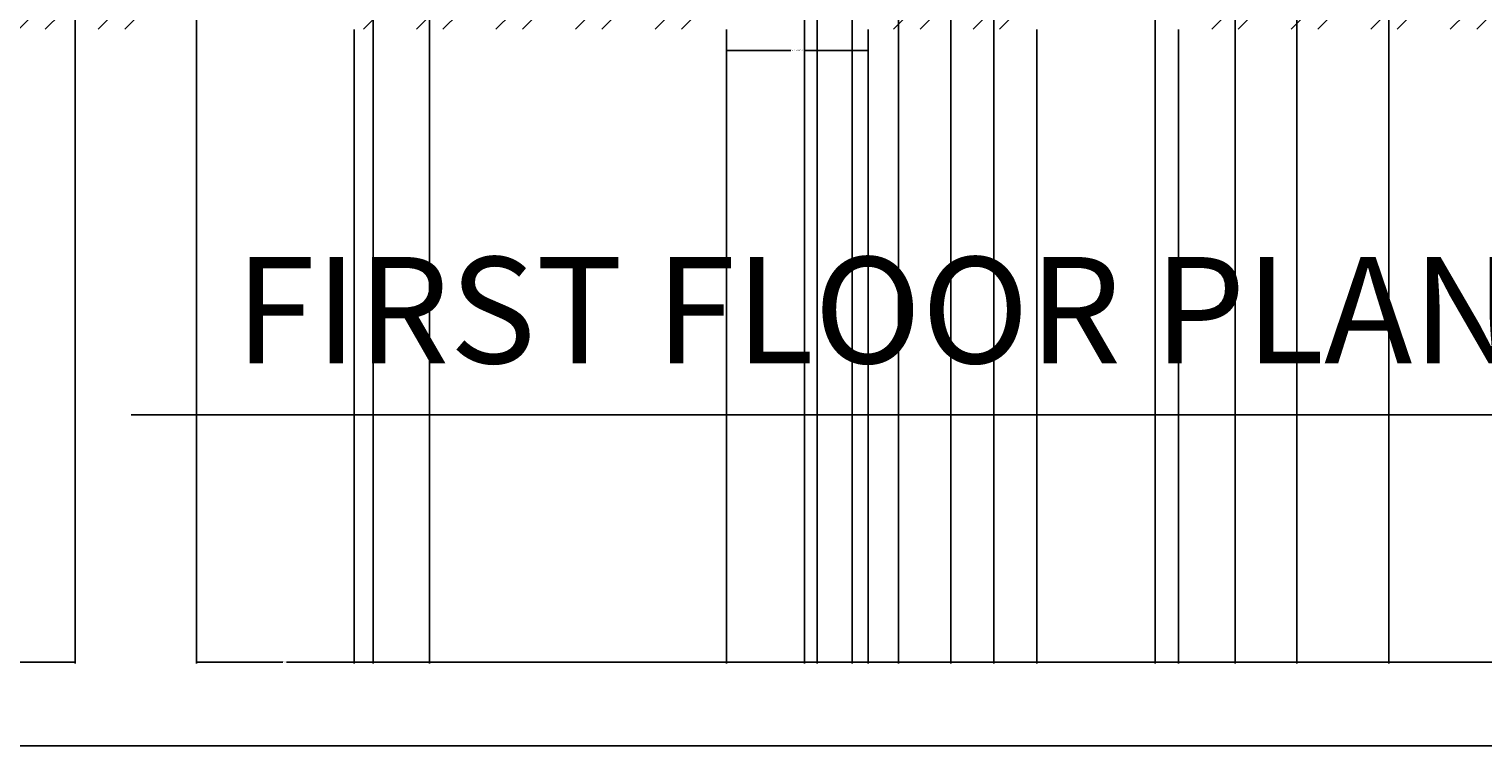
# Model space of a CAD drawing. Units: inches. Extents: x 1748 to 2382, y 1346 to 2284.
# Tile 2 of 26: x 1901 to 2147, y 1346 to 1468. Entities that reach past the tile are written whole.
import ezdxf

# ---------------------------------------------------------------- set-up
doc = ezdxf.new("R2010")
doc.units = ezdxf.units.IN
for name, color, linetype, lineweight in [('A-ANNO-DIMS', 2, 'Continuous', 18), ('A-ANNO-TTLB', 7, 'Continuous', 25), ('A-WALL-PATT', 9, 'Continuous', 13)]:
    doc.layers.add(name, color=color, linetype=linetype, lineweight=lineweight)
doc.styles.get("Standard").update_dxf_attribs({"font": 'arial.ttf'})
doc.dimstyles.get("Standard").update_dxf_attribs({"dimtxt": 0.18, "dimasz": 0.18, "dimexe": 0.18, "dimexo": 0.0625, "dimgap": 0.09, "dimtad": 0, "dimtih": 1, "dimtoh": 1, "dimdec": 4, "dimzin": 0, "dimdsep": 46, "dimtxsty": 'Standard', "dimcen": 0.09, "dimadec": 0, "dimazin": 0, "dimtfac": 1, "dimtdec": 4, "dimtofl": 0, "dimtmove": 0, "dimatfit": 3, "dimfxl": 1, "dimtolj": 1, "dimtzin": 0, "dimarcsym": 0})

# ---------------------------------------------------------------- blocks, each defined once
blk = doc.blocks.new('*D32')
at = {"layer": 'A-ANNO-DIMS', "color": 0, "lineweight": -2, "transparency": 16777216}
for p, q in [((2018.79, 1467.79), (2018.79, 1464.07)), ((2042.79, 1467.79), (2042.79, 1464.07)), ((2018.97, 1464.25), (2029.67, 1464.25)), ((2042.61, 1464.25), (2031.91, 1464.25))]:
    blk.add_line(p, q, dxfattribs=at)
at = {"layer": 'A-ANNO-DIMS', "color": 0, "transparency": 16777216}
for points in [[(2018.97, 1464.28), (2018.97, 1464.22), (2018.79, 1464.25)], [(2042.61, 1464.28), (2042.61, 1464.22), (2042.79, 1464.25)]]:
    blk.add_solid(points, dxfattribs=at)
at = {"layer": 'Defpoints', "color": 0, "transparency": 16777216}
for p in [(2018.79, 1467.85), (2042.79, 1467.85), (2042.79, 1464.25)]:
    blk.add_point(p, dxfattribs=at)
at = {"layer": 'A-ANNO-DIMS', "color": 0, "transparency": 16777216, "insert": (2030.79, 1464.25), "char_height": 0.18, "attachment_point": 5}
blk.add_mtext('\\A1;WINDOW 24 TYP.', dxfattribs=at)
blk = doc.blocks.new('*D36')
at = {"layer": 'A-ANNO-DIMS', "color": 0, "lineweight": -2, "transparency": 16777216}
for p, q in [((2031.96, 1970.29), (2031.96, 1360.47)), ((2130.96, 1970.29), (2130.96, 1360.47)), ((2032.14, 1360.65), (2081.24, 1360.65)), ((2130.78, 1360.65), (2081.68, 1360.65))]:
    blk.add_line(p, q, dxfattribs=at)
at = {"layer": 'A-ANNO-DIMS', "color": 0, "transparency": 16777216}
for points in [[(2032.14, 1360.68), (2032.14, 1360.62), (2031.96, 1360.65)], [(2130.78, 1360.68), (2130.78, 1360.62), (2130.96, 1360.65)]]:
    blk.add_solid(points, dxfattribs=at)
at = {"layer": 'Defpoints', "color": 0, "transparency": 16777216}
for p in [(2031.96, 1970.35), (2130.96, 1970.35), (2130.96, 1360.65)]:
    blk.add_point(p, dxfattribs=at)
at = {"layer": 'A-ANNO-DIMS', "color": 0, "transparency": 16777216, "insert": (2081.46, 1360.65), "char_height": 0.18, "attachment_point": 5}
blk.add_mtext('\\A1;99', dxfattribs=at)
blk = doc.blocks.new('*D50')
at = {"layer": 'A-ANNO-DIMS', "color": 0, "lineweight": -2, "transparency": 16777216}
for p, q in [((1869.96, 2223.79), (1869.96, 1360.47)), ((1908.44, 2223.79), (1908.44, 1360.47)), ((1870.14, 1360.65), (1888.81, 1360.65)), ((1908.26, 1360.65), (1889.6, 1360.65))]:
    blk.add_line(p, q, dxfattribs=at)
at = {"layer": 'A-ANNO-DIMS', "color": 0, "transparency": 16777216}
for points in [[(1870.14, 1360.68), (1870.14, 1360.62), (1869.96, 1360.65)], [(1908.26, 1360.68), (1908.26, 1360.62), (1908.44, 1360.65)]]:
    blk.add_solid(points, dxfattribs=at)
at = {"layer": 'Defpoints', "color": 0, "transparency": 16777216}
for p in [(1869.96, 2223.85), (1908.44, 2223.85), (1908.44, 1360.65)]:
    blk.add_point(p, dxfattribs=at)
at = {"layer": 'A-ANNO-DIMS', "color": 0, "transparency": 16777216, "insert": (1889.2, 1360.65), "char_height": 0.18, "attachment_point": 5}
blk.add_mtext('\\A1;38.48', dxfattribs=at)
blk = doc.blocks.new('*D51')
at = {"layer": 'A-ANNO-DIMS', "color": 0, "lineweight": -2, "transparency": 16777216}
for p, q in [((1968.44, 2223.79), (1968.44, 1360.47)), ((2040.07, 2223.79), (2040.07, 1360.47)), ((1968.62, 1360.65), (2003.86, 1360.65)), ((2039.89, 1360.65), (2004.65, 1360.65))]:
    blk.add_line(p, q, dxfattribs=at)
at = {"layer": 'A-ANNO-DIMS', "color": 0, "transparency": 16777216}
for points in [[(1968.62, 1360.68), (1968.62, 1360.62), (1968.44, 1360.65)], [(2039.89, 1360.68), (2039.89, 1360.62), (2040.07, 1360.65)]]:
    blk.add_solid(points, dxfattribs=at)
at = {"layer": 'Defpoints', "color": 0, "transparency": 16777216}
for p in [(1968.44, 2223.85), (2040.07, 2223.85), (2040.07, 1360.65)]:
    blk.add_point(p, dxfattribs=at)
at = {"layer": 'A-ANNO-DIMS', "color": 0, "transparency": 16777216, "insert": (2004.26, 1360.65), "char_height": 0.18, "attachment_point": 5}
blk.add_mtext('\\A1;71.62', dxfattribs=at)
blk = doc.blocks.new('*D52')
at = {"layer": 'A-ANNO-DIMS', "color": 0, "lineweight": -2, "transparency": 16777216}
for p, q in [((2064.07, 2223.79), (2064.07, 1360.47)), ((2091.4, 2223.79), (2091.4, 1360.47)), ((2064.25, 1360.65), (2077.34, 1360.65)), ((2091.22, 1360.65), (2078.13, 1360.65))]:
    blk.add_line(p, q, dxfattribs=at)
at = {"layer": 'A-ANNO-DIMS', "color": 0, "transparency": 16777216}
for points in [[(2064.25, 1360.68), (2064.25, 1360.62), (2064.07, 1360.65)], [(2091.22, 1360.68), (2091.22, 1360.62), (2091.4, 1360.65)]]:
    blk.add_solid(points, dxfattribs=at)
at = {"layer": 'Defpoints', "color": 0, "transparency": 16777216}
for p in [(2064.07, 2223.85), (2091.4, 2223.85), (2091.4, 1360.65)]:
    blk.add_point(p, dxfattribs=at)
at = {"layer": 'A-ANNO-DIMS', "color": 0, "transparency": 16777216, "insert": (2077.73, 1360.65), "char_height": 0.18, "attachment_point": 5}
blk.add_mtext('\\A1;27.33', dxfattribs=at)
blk = doc.blocks.new('*D53')
at = {"layer": 'A-ANNO-DIMS', "color": 0, "lineweight": -2, "transparency": 16777216}
for p, q in [((2115.4, 2223.79), (2115.4, 1360.47)), ((2167.02, 2223.79), (2167.02, 1360.47)), ((2115.58, 1360.65), (2140.81, 1360.65)), ((2166.84, 1360.65), (2141.6, 1360.65))]:
    blk.add_line(p, q, dxfattribs=at)
at = {"layer": 'A-ANNO-DIMS', "color": 0, "transparency": 16777216}
for points in [[(2115.58, 1360.68), (2115.58, 1360.62), (2115.4, 1360.65)], [(2166.84, 1360.68), (2166.84, 1360.62), (2167.02, 1360.65)]]:
    blk.add_solid(points, dxfattribs=at)
at = {"layer": 'Defpoints', "color": 0, "transparency": 16777216}
for p in [(2115.4, 2223.85), (2167.02, 2223.85), (2167.02, 1360.65)]:
    blk.add_point(p, dxfattribs=at)
at = {"layer": 'A-ANNO-DIMS', "color": 0, "transparency": 16777216, "insert": (2141.21, 1360.65), "char_height": 0.18, "attachment_point": 5}
blk.add_mtext('\\A1;51.62', dxfattribs=at)
blk = doc.blocks.new('*D61')
at = {"layer": 'A-ANNO-DIMS', "color": 0, "lineweight": -2, "transparency": 16777216}
for p, q in [((2047.92, 1854.79), (2047.92, 1360.47)), ((2104.96, 1854.79), (2104.96, 1360.47)), ((2048.1, 1360.65), (2076.04, 1360.65)), ((2104.78, 1360.65), (2076.83, 1360.65))]:
    blk.add_line(p, q, dxfattribs=at)
at = {"layer": 'A-ANNO-DIMS', "color": 0, "transparency": 16777216}
for points in [[(2048.1, 1360.68), (2048.1, 1360.62), (2047.92, 1360.65)], [(2104.78, 1360.68), (2104.78, 1360.62), (2104.96, 1360.65)]]:
    blk.add_solid(points, dxfattribs=at)
at = {"layer": 'Defpoints', "color": 0, "transparency": 16777216}
for p in [(2047.92, 1854.85), (2104.96, 1854.85), (2104.96, 1360.65)]:
    blk.add_point(p, dxfattribs=at)
at = {"layer": 'A-ANNO-DIMS', "color": 0, "transparency": 16777216, "insert": (2076.44, 1360.65), "char_height": 0.18, "attachment_point": 5}
blk.add_mtext('\\A1;57.04', dxfattribs=at)
blk = doc.blocks.new('*D65')
at = {"layer": 'A-ANNO-DIMS', "color": 0, "lineweight": -2, "transparency": 16777216}
for p, q in [((1955.68, 1467.79), (1955.68, 1360.47)), ((2018.79, 1467.79), (2018.79, 1360.47)), ((1955.86, 1360.65), (1986.86, 1360.65)), ((2018.61, 1360.65), (1987.61, 1360.65))]:
    blk.add_line(p, q, dxfattribs=at)
at = {"layer": 'A-ANNO-DIMS', "color": 0, "transparency": 16777216}
for points in [[(1955.86, 1360.68), (1955.86, 1360.62), (1955.68, 1360.65)], [(2018.61, 1360.68), (2018.61, 1360.62), (2018.79, 1360.65)]]:
    blk.add_solid(points, dxfattribs=at)
at = {"layer": 'Defpoints', "color": 0, "transparency": 16777216}
for p in [(1955.68, 1467.85), (2018.79, 1467.85), (2018.79, 1360.65)]:
    blk.add_point(p, dxfattribs=at)
at = {"layer": 'A-ANNO-DIMS', "color": 0, "transparency": 16777216, "insert": (1987.23, 1360.65), "char_height": 0.18, "attachment_point": 5}
blk.add_mtext('\\A1;63.11', dxfattribs=at)
blk = doc.blocks.new('*D66')
at = {"layer": 'A-ANNO-DIMS', "color": 0, "lineweight": -2, "transparency": 16777216}
for p, q in [((2042.79, 1467.79), (2042.79, 1360.47)), ((2071.36, 1467.79), (2071.36, 1360.47)), ((2042.97, 1360.65), (2056.61, 1360.65)), ((2071.18, 1360.65), (2057.54, 1360.65))]:
    blk.add_line(p, q, dxfattribs=at)
at = {"layer": 'A-ANNO-DIMS', "color": 0, "transparency": 16777216}
for points in [[(2042.97, 1360.68), (2042.97, 1360.62), (2042.79, 1360.65)], [(2071.18, 1360.68), (2071.18, 1360.62), (2071.36, 1360.65)]]:
    blk.add_solid(points, dxfattribs=at)
at = {"layer": 'Defpoints', "color": 0, "transparency": 16777216}
for p in [(2042.79, 1467.85), (2071.36, 1467.85), (2071.36, 1360.65)]:
    blk.add_point(p, dxfattribs=at)
at = {"layer": 'A-ANNO-DIMS', "color": 0, "transparency": 16777216, "insert": (2057.07, 1360.65), "char_height": 0.18, "attachment_point": 5}
blk.add_mtext('\\A1;28.574', dxfattribs=at)
blk = doc.blocks.new('*D67')
at = {"layer": 'A-ANNO-DIMS', "color": 0, "lineweight": -2, "transparency": 16777216}
for p, q in [((2095.36, 1467.79), (2095.36, 1360.47)), ((2152.34, 1467.79), (2152.34, 1360.47)), ((2095.54, 1360.65), (2123.45, 1360.65)), ((2152.16, 1360.65), (2124.24, 1360.65))]:
    blk.add_line(p, q, dxfattribs=at)
at = {"layer": 'A-ANNO-DIMS', "color": 0, "transparency": 16777216}
for points in [[(2095.54, 1360.68), (2095.54, 1360.62), (2095.36, 1360.65)], [(2152.16, 1360.68), (2152.16, 1360.62), (2152.34, 1360.65)]]:
    blk.add_solid(points, dxfattribs=at)
at = {"layer": 'Defpoints', "color": 0, "transparency": 16777216}
for p in [(2095.36, 1467.85), (2152.34, 1467.85), (2152.34, 1360.65)]:
    blk.add_point(p, dxfattribs=at)
at = {"layer": 'A-ANNO-DIMS', "color": 0, "transparency": 16777216, "insert": (2123.85, 1360.65), "char_height": 0.18, "attachment_point": 5}
blk.add_mtext('\\A1;56.97', dxfattribs=at)
blk = doc.blocks.new('*D78')
at = {"layer": 'A-ANNO-DIMS', "color": 0, "lineweight": -2, "transparency": 16777216}
for p, q in [((2034.13, 2132.54), (2034.13, 1360.47)), ((2056.8, 2127.06), (2056.8, 1360.47)), ((2034.31, 1360.65), (2045, 1360.65)), ((2056.62, 1360.65), (2045.93, 1360.65))]:
    blk.add_line(p, q, dxfattribs=at)
at = {"layer": 'A-ANNO-DIMS', "color": 0, "transparency": 16777216}
for points in [[(2034.31, 1360.68), (2034.31, 1360.62), (2034.13, 1360.65)], [(2056.62, 1360.68), (2056.62, 1360.62), (2056.8, 1360.65)]]:
    blk.add_solid(points, dxfattribs=at)
at = {"layer": 'Defpoints', "color": 0, "transparency": 16777216}
for p in [(2034.13, 2132.6), (2056.8, 2127.13), (2056.8, 1360.65)]:
    blk.add_point(p, dxfattribs=at)
at = {"layer": 'A-ANNO-DIMS', "color": 0, "transparency": 16777216, "insert": (2045.47, 1360.65), "char_height": 0.18, "attachment_point": 5}
blk.add_mtext('\\A1;22.663', dxfattribs=at)
blk = doc.blocks.new('*D79')
at = {"layer": 'A-ANNO-DIMS', "color": 0, "lineweight": -2, "transparency": 16777216}
for p, q in [((1929, 1854.79), (1929, 1360.47)), ((1958.9, 1854.79), (1958.9, 1360.47)), ((1929.18, 1360.65), (1943.62, 1360.65)), ((1958.72, 1360.65), (1944.27, 1360.65))]:
    blk.add_line(p, q, dxfattribs=at)
at = {"layer": 'A-ANNO-DIMS', "color": 0, "transparency": 16777216}
for points in [[(1929.18, 1360.68), (1929.18, 1360.62), (1929, 1360.65)], [(1958.72, 1360.68), (1958.72, 1360.62), (1958.9, 1360.65)]]:
    blk.add_solid(points, dxfattribs=at)
at = {"layer": 'Defpoints', "color": 0, "transparency": 16777216}
for p in [(1929, 1854.85), (1958.9, 1854.85), (1958.9, 1360.65)]:
    blk.add_point(p, dxfattribs=at)
at = {"layer": 'A-ANNO-DIMS', "color": 0, "transparency": 16777216, "insert": (1943.95, 1360.65), "char_height": 0.18, "attachment_point": 5}
blk.add_mtext('\\A1;29.9', dxfattribs=at)

msp = doc.modelspace()

# ---------------------------------------------------------------- hatches: boundary and pattern name
at = {"layer": 'A-WALL-PATT'}
h = msp.add_hatch(dxfattribs=at)
h.set_pattern_fill('ANSI32', color=256)
h.paths.add_polyline_path([(1908.4445, 2232.8497), (1821.9607, 2232.8497), (1821.9607, 2223.8497), (1865.4607, 2223.8497), (1865.4607, 2209.9185), (1869.9607, 2209.9185), (1869.9607, 2223.8497), (1908.4445, 2223.8497), (1908.4445, 2228.3497)])
h.paths.add_polyline_path([(2040.0683, 2232.8497), (1968.4445, 2232.8497), (1968.4445, 2223.8497), (2025.9607, 2223.8497), (2025.9607, 2130.3497), (2032.1341, 2130.3497), (2032.1341, 2132.5997), (2032.1341, 2134.8497), (2030.4607, 2134.8497), (2030.4607, 2223.8497), (2040.0683, 2223.8497)])
h.paths.add_polyline_path([(2091.3969, 2232.8497), (2064.0683, 2232.8497), (2064.0683, 2223.8497), (2078.4607, 2223.8497), (2078.4607, 2134.8497), (2051.1563, 2134.8497), (2051.1563, 2130.3497), (2078.4607, 2130.3497), (2078.4607, 2128.6813), (2082.9607, 2128.6813), (2082.9607, 2130.3497), (2086.1879, 2130.3497), (2086.1879, 2132.5997), (2086.1879, 2134.8497), (2082.9607, 2134.8497), (2082.9607, 2223.8497), (2091.3969, 2223.8497), (2091.3969, 2228.3497)])
h.paths.add_polyline_path([(2167.0164, 2232.8497), (2115.3969, 2232.8497), (2115.3969, 2223.8497), (2130.9607, 2223.8497), (2130.9607, 2134.8497), (2106.9607, 2134.8497), (2106.9607, 2130.3497), (2135.4607, 2130.3497), (2135.4607, 2223.8497), (2167.0164, 2223.8497), (2167.0164, 2228.3497)])
h.paths.add_polyline_path([(1869.9607, 2149.9185), (1865.4607, 2149.9185), (1865.4607, 2127.8942), (1869.9607, 2127.8942)])
h.paths.add_polyline_path([(2082.9607, 2104.4871), (2080.7107, 2104.4871), (2078.4607, 2104.4871), (2078.4607, 2103.8497), (1869.9607, 2103.8497), (1869.9607, 2108.6062), (1867.7107, 2108.6062), (1865.4607, 2108.6062), (1865.4607, 2103.8497), (1821.9607, 2103.8497), (1821.9607, 2099.3497), (1865.4607, 2099.3497), (1865.4607, 2094.7509), (1869.9607, 2094.7509), (1869.9607, 2099.3497), (2025.9607, 2099.3497), (2025.9607, 2096.4326), (2030.4607, 2096.4326), (2030.4607, 2099.3497), (2082.9607, 2099.3497)])
h.paths.add_polyline_path([(1928.9457, 1401.1212), (2176.8693, 1401.1212), (2176.8693, 1438.214), (1928.9457, 1438.214)], flags=9)
h.paths.add_polyline_path([(2122.2668, 2048.1927), (2177.9387, 2048.1927), (2177.9387, 2066.85), (2122.2668, 2066.85)], flags=9)
h.paths.add_polyline_path([(2272.688, 2153.8197), (2272.688, 2216.746), (2262.3845, 2216.746), (2262.3845, 2153.8197)], flags=9)
h.paths.add_polyline_path([(2157.2928, 2166.5593), (2196.3822, 2166.5593), (2196.3822, 2185.2167), (2157.2928, 2185.2167)], flags=9)
h.paths.add_polyline_path([(2089.3407, 2162.0698), (2124.3987, 2162.0698), (2124.3987, 2180.7272), (2089.3407, 2180.7272)], flags=9)
h.paths.add_polyline_path([(2037.4521, 2160.0913), (2072.5101, 2160.0913), (2072.5101, 2178.7486), (2037.4521, 2178.7486)], flags=9)
h.paths.add_polyline_path([(1884.7894, 2104.1554), (1923.6297, 2104.1554), (1923.6297, 2122.8127), (1884.7894, 2122.8127)], flags=9)
h.paths.add_polyline_path([(1851.2832, 2142.9749), (1851.2832, 2199.3051), (1840.9796, 2199.3051), (1840.9796, 2142.9749)], flags=9)
h.paths.add_polyline_path([(1844.8763, 2017.2834), (1844.8763, 2073.6136), (1834.5728, 2073.6136), (1834.5728, 2017.2834)], flags=9)
h.paths.add_polyline_path([(1897.1577, 2073.1279), (1935.9981, 2073.1279), (1935.9981, 2091.7853), (1897.1577, 2091.7853)], flags=9)
h.paths.add_polyline_path([(1952.3395, 1802.4231), (2008.0114, 1802.4231), (2008.0114, 1821.0805), (1952.3395, 1821.0805)], flags=9)
h.paths.add_polyline_path([(1978.8184, 1857.6841), (2017.7338, 1857.6841), (2017.7338, 1876.3415), (1978.8184, 1876.3415)], flags=9)
h.paths.add_polyline_path([(1979.6513, 1925.9516), (2008.8089, 1925.9516), (2008.8089, 1944.6089), (1979.6513, 1944.6089)], flags=9)
h.paths.add_polyline_path([(1838.5553, 1860.3527), (1877.3957, 1860.3527), (1877.3957, 1879.01), (1838.5553, 1879.01)], flags=9)
h.paths.add_polyline_path([(1883.9018, 1787.3013), (1883.9018, 1843.6315), (1873.5983, 1843.6315), (1873.5983, 1787.3013)], flags=9)
h.paths.add_polyline_path([(1873.7079, 1509.1938), (1873.7079, 1583.7709), (1863.4044, 1583.7709), (1863.4044, 1509.1938)], flags=9)
h.paths.add_polyline_path([(1916.2259, 1603.3681), (1955.0663, 1603.3681), (1955.0663, 1622.0254), (1916.2259, 1622.0254)], flags=9)
h.paths.add_polyline_path([(1876.3013, 1636.757), (1876.3013, 1693.0871), (1865.9978, 1693.0871), (1865.9978, 1636.757)], flags=9)
h.paths.add_polyline_path([(1921.3138, 1521.8316), (1964.0662, 1521.8316), (1964.0662, 1540.489), (1921.3138, 1540.489)], flags=9)
h.paths.add_polyline_path([(2017.5657, 1497.5078), (2046.7983, 1497.5078), (2046.7983, 1516.1651), (2017.5657, 1516.1651)], flags=9)
h.paths.add_polyline_path([(2066.8661, 1499.3902), (2096.0988, 1499.3902), (2096.0988, 1518.0475), (2066.8661, 1518.0475)], flags=9)
h.paths.add_polyline_path([(2155.4835, 1571.6596), (2198.2358, 1571.6596), (2198.2358, 1590.3169), (2155.4835, 1590.3169)], flags=9)
h.paths.add_polyline_path([(2094.9136, 1664.6812), (2150.5855, 1664.6812), (2150.5855, 1683.3386), (2094.9136, 1683.3386)], flags=9)
h.paths.add_polyline_path([(2257.6902, 1863.1628), (2269.8935, 1863.1628), (2269.8935, 1873.4664), (2257.6902, 1873.4664)], flags=9)
h.paths.add_polyline_path([(2164.0748, 1880.3089), (2189.8694, 1880.3089), (2189.8694, 1890.6124), (2164.0748, 1890.6124)], flags=9)
h.paths.add_polyline_path([(2239.4394, 1931.0585), (2268.8187, 1931.0585), (2268.8187, 1949.7159), (2239.4394, 1949.7159)], flags=9)
h = msp.add_hatch(dxfattribs=at)
h.set_pattern_fill('ANSI32', color=256)
h.paths.add_polyline_path([(2297.4607, 2232.8497), (2203.0164, 2232.8497), (2203.0164, 2223.8497), (2244.9607, 2223.8497), (2244.9607, 2127.8554), (2249.4607, 2127.8554), (2249.4607, 2223.8497), (2297.4607, 2223.8497)])
h.paths.add_polyline_path([(2297.4607, 2103.8497), (2249.4607, 2103.8497), (2249.4607, 2106.7497), (2247.2107, 2106.7497), (2244.9607, 2106.7497), (2244.9607, 2103.8497), (2130.9607, 2103.8497), (2130.9607, 2099.3497), (2288.4607, 2099.3497), (2288.4607, 2077.2008), (2297.4607, 2077.2008)])
h.paths.add_polyline_path([(1928.9457, 1401.1212), (2176.8693, 1401.1212), (2176.8693, 1438.214), (1928.9457, 1438.214)], flags=9)
h.paths.add_polyline_path([(2122.2668, 2048.1927), (2177.9387, 2048.1927), (2177.9387, 2066.85), (2122.2668, 2066.85)], flags=9)
h.paths.add_polyline_path([(2272.688, 2153.8197), (2272.688, 2216.746), (2262.3845, 2216.746), (2262.3845, 2153.8197)], flags=25)
h.paths.add_polyline_path([(2157.2928, 2166.5593), (2196.3822, 2166.5593), (2196.3822, 2185.2167), (2157.2928, 2185.2167)], flags=9)
h.paths.add_polyline_path([(2089.3407, 2162.0698), (2124.3987, 2162.0698), (2124.3987, 2180.7272), (2089.3407, 2180.7272)], flags=9)
h.paths.add_polyline_path([(2037.4521, 2160.0913), (2072.5101, 2160.0913), (2072.5101, 2178.7486), (2037.4521, 2178.7486)], flags=9)
h.paths.add_polyline_path([(1884.7894, 2104.1554), (1923.6297, 2104.1554), (1923.6297, 2122.8127), (1884.7894, 2122.8127)], flags=9)
h.paths.add_polyline_path([(1851.2832, 2142.9749), (1851.2832, 2199.3051), (1840.9796, 2199.3051), (1840.9796, 2142.9749)], flags=9)
h.paths.add_polyline_path([(1844.8763, 2017.2834), (1844.8763, 2073.6136), (1834.5728, 2073.6136), (1834.5728, 2017.2834)], flags=9)
h.paths.add_polyline_path([(1897.1577, 2073.1279), (1935.9981, 2073.1279), (1935.9981, 2091.7853), (1897.1577, 2091.7853)], flags=9)
h.paths.add_polyline_path([(1952.3395, 1802.4231), (2008.0114, 1802.4231), (2008.0114, 1821.0805), (1952.3395, 1821.0805)], flags=9)
h.paths.add_polyline_path([(1978.8184, 1857.6841), (2017.7338, 1857.6841), (2017.7338, 1876.3415), (1978.8184, 1876.3415)], flags=9)
h.paths.add_polyline_path([(1979.6513, 1925.9516), (2008.8089, 1925.9516), (2008.8089, 1944.6089), (1979.6513, 1944.6089)], flags=9)
h.paths.add_polyline_path([(1838.5553, 1860.3527), (1877.3957, 1860.3527), (1877.3957, 1879.01), (1838.5553, 1879.01)], flags=9)
h.paths.add_polyline_path([(1883.9018, 1787.3013), (1883.9018, 1843.6315), (1873.5983, 1843.6315), (1873.5983, 1787.3013)], flags=9)
h.paths.add_polyline_path([(1873.7079, 1509.1938), (1873.7079, 1583.7709), (1863.4044, 1583.7709), (1863.4044, 1509.1938)], flags=9)
h.paths.add_polyline_path([(1916.2259, 1603.3681), (1955.0663, 1603.3681), (1955.0663, 1622.0254), (1916.2259, 1622.0254)], flags=9)
h.paths.add_polyline_path([(1876.3013, 1636.757), (1876.3013, 1693.0871), (1865.9978, 1693.0871), (1865.9978, 1636.757)], flags=9)
h.paths.add_polyline_path([(1921.3138, 1521.8316), (1964.0662, 1521.8316), (1964.0662, 1540.489), (1921.3138, 1540.489)], flags=9)
h.paths.add_polyline_path([(2017.5657, 1497.5078), (2046.7983, 1497.5078), (2046.7983, 1516.1651), (2017.5657, 1516.1651)], flags=9)
h.paths.add_polyline_path([(2066.8661, 1499.3902), (2096.0988, 1499.3902), (2096.0988, 1518.0475), (2066.8661, 1518.0475)], flags=9)
h.paths.add_polyline_path([(2155.4835, 1571.6596), (2198.2358, 1571.6596), (2198.2358, 1590.3169), (2155.4835, 1590.3169)], flags=9)
h.paths.add_polyline_path([(2094.9136, 1664.6812), (2150.5855, 1664.6812), (2150.5855, 1683.3386), (2094.9136, 1683.3386)], flags=9)
h.paths.add_polyline_path([(2257.6902, 1863.1628), (2269.8935, 1863.1628), (2269.8935, 1873.4664), (2257.6902, 1873.4664)], flags=9)
h.paths.add_polyline_path([(2164.0748, 1880.3089), (2189.8694, 1880.3089), (2189.8694, 1890.6124), (2164.0748, 1890.6124)], flags=9)
h.paths.add_polyline_path([(2239.4394, 1931.0585), (2268.8187, 1931.0585), (2268.8187, 1949.7159), (2239.4394, 1949.7159)], flags=9)
h = msp.add_hatch(dxfattribs=at)
h.set_pattern_fill('ANSI32', color=256)
h.paths.add_polyline_path([(1919.6777, 1476.8497), (1900.6426, 1476.8497), (1900.6426, 1522.0826), (1898.3926, 1522.0826), (1896.1426, 1522.0826), (1896.1426, 1476.8497), (1857.1426, 1476.8497), (1857.1426, 1467.8497), (1896.1426, 1467.8497), (1919.6777, 1467.8497), (1919.6777, 1472.3497)])
h.paths.add_polyline_path([(2018.7873, 1472.3497), (2018.7873, 1476.8497), (2010.9607, 1476.8497), (2010.9607, 1560.8497), (2034.9607, 1560.8497), (2034.9607, 1565.3497), (2006.4607, 1565.3497), (2006.4607, 1476.8497), (1955.6777, 1476.8497), (1955.6777, 1467.8497), (2018.7873, 1467.8497)])
h.paths.add_polyline_path([(2152.3354, 1472.3497), (2152.3354, 1476.8497), (2115.9607, 1476.8497), (2115.9607, 1565.3497), (2109.2204, 1565.3497), (2109.2204, 1563.0997), (2109.2204, 1560.8497), (2111.4607, 1560.8497), (2111.4607, 1476.8497), (2095.3617, 1476.8497), (2095.3617, 1467.8497), (2152.3354, 1467.8497)])
h.paths.add_polyline_path([(2071.3617, 1476.8497), (2063.4607, 1476.8497), (2063.4607, 1560.8497), (2090.1865, 1560.8497), (2090.1865, 1565.3497), (2063.4607, 1565.3497), (2063.4607, 1572.5485), (2061.2107, 1572.5485), (2058.9607, 1572.5485), (2058.9607, 1565.3497), (2055.6281, 1565.3497), (2055.6281, 1560.8497), (2058.9607, 1560.8497), (2058.9607, 1476.8497), (2042.7873, 1476.8497), (2042.7873, 1467.8497), (2071.3617, 1467.8497), (2071.3617, 1472.3497)])
h.paths.add_polyline_path([(2297.4607, 1506.5652), (2288.4607, 1506.5652), (2288.4607, 1476.8497), (2212.3354, 1476.8497), (2212.3354, 1467.8497), (2297.4607, 1467.8497)])
h.paths.add_polyline_path([(2297.4607, 1645.3038), (2288.4607, 1645.3038), (2288.4607, 1605.8497), (2058.9607, 1605.8497), (2058.9607, 1600.1857), (2061.2107, 1600.1857), (2063.4607, 1600.1857), (2063.4607, 1601.3497), (2288.4607, 1601.3497), (2288.4607, 1566.5652), (2297.4607, 1566.5652)])
h.paths.add_polyline_path([(2010.9607, 1609.0561), (2008.7107, 1609.0561), (2006.4607, 1609.0561), (2006.4607, 1605.8497), (1900.6426, 1605.8497), (1900.6426, 1609.7171), (1898.3926, 1609.7171), (1896.1426, 1609.7171), (1896.1426, 1605.8497), (1857.1426, 1605.8497), (1857.1426, 1601.3497), (1896.1426, 1601.3497), (1896.1426, 1542.5447), (1900.6426, 1542.5447), (1900.6426, 1601.3497), (2010.9607, 1601.3497)])
h.paths.add_polyline_path([(1928.9457, 1401.1212), (2176.8693, 1401.1212), (2176.8693, 1438.214), (1928.9457, 1438.214)], flags=9)
h.paths.add_polyline_path([(2122.2668, 2048.1927), (2177.9387, 2048.1927), (2177.9387, 2066.85), (2122.2668, 2066.85)], flags=9)
h.paths.add_polyline_path([(2272.688, 2153.8197), (2272.688, 2216.746), (2262.3845, 2216.746), (2262.3845, 2153.8197)], flags=9)
h.paths.add_polyline_path([(2157.2928, 2166.5593), (2196.3822, 2166.5593), (2196.3822, 2185.2167), (2157.2928, 2185.2167)], flags=9)
h.paths.add_polyline_path([(2089.3407, 2162.0698), (2124.3987, 2162.0698), (2124.3987, 2180.7272), (2089.3407, 2180.7272)], flags=9)
h.paths.add_polyline_path([(2037.4521, 2160.0913), (2072.5101, 2160.0913), (2072.5101, 2178.7486), (2037.4521, 2178.7486)], flags=9)
h.paths.add_polyline_path([(1884.7894, 2104.1554), (1923.6297, 2104.1554), (1923.6297, 2122.8127), (1884.7894, 2122.8127)], flags=9)
h.paths.add_polyline_path([(1851.2832, 2142.9749), (1851.2832, 2199.3051), (1840.9796, 2199.3051), (1840.9796, 2142.9749)], flags=9)
h.paths.add_polyline_path([(1844.8763, 2017.2834), (1844.8763, 2073.6136), (1834.5728, 2073.6136), (1834.5728, 2017.2834)], flags=9)
h.paths.add_polyline_path([(1897.1577, 2073.1279), (1935.9981, 2073.1279), (1935.9981, 2091.7853), (1897.1577, 2091.7853)], flags=9)
h.paths.add_polyline_path([(1952.3395, 1802.4231), (2008.0114, 1802.4231), (2008.0114, 1821.0805), (1952.3395, 1821.0805)], flags=9)
h.paths.add_polyline_path([(1978.8184, 1857.6841), (2017.7338, 1857.6841), (2017.7338, 1876.3415), (1978.8184, 1876.3415)], flags=9)
h.paths.add_polyline_path([(1979.6513, 1925.9516), (2008.8089, 1925.9516), (2008.8089, 1944.6089), (1979.6513, 1944.6089)], flags=9)
h.paths.add_polyline_path([(1838.5553, 1860.3527), (1877.3957, 1860.3527), (1877.3957, 1879.01), (1838.5553, 1879.01)], flags=9)
h.paths.add_polyline_path([(1883.9018, 1787.3013), (1883.9018, 1843.6315), (1873.5983, 1843.6315), (1873.5983, 1787.3013)], flags=9)
h.paths.add_polyline_path([(1873.7079, 1509.1938), (1873.7079, 1583.7709), (1863.4044, 1583.7709), (1863.4044, 1509.1938)], flags=9)
h.paths.add_polyline_path([(1916.2259, 1603.3681), (1955.0663, 1603.3681), (1955.0663, 1622.0254), (1916.2259, 1622.0254)], flags=9)
h.paths.add_polyline_path([(1876.3013, 1636.757), (1876.3013, 1693.0871), (1865.9978, 1693.0871), (1865.9978, 1636.757)], flags=9)
h.paths.add_polyline_path([(1921.3138, 1521.8316), (1964.0662, 1521.8316), (1964.0662, 1540.489), (1921.3138, 1540.489)], flags=9)
h.paths.add_polyline_path([(2017.5657, 1497.5078), (2046.7983, 1497.5078), (2046.7983, 1516.1651), (2017.5657, 1516.1651)], flags=9)
h.paths.add_polyline_path([(2066.8661, 1499.3902), (2096.0988, 1499.3902), (2096.0988, 1518.0475), (2066.8661, 1518.0475)], flags=9)
h.paths.add_polyline_path([(2155.4835, 1571.6596), (2198.2358, 1571.6596), (2198.2358, 1590.3169), (2155.4835, 1590.3169)], flags=25)
h.paths.add_polyline_path([(2094.9136, 1664.6812), (2150.5855, 1664.6812), (2150.5855, 1683.3386), (2094.9136, 1683.3386)], flags=9)
h.paths.add_polyline_path([(2257.6902, 1863.1628), (2269.8935, 1863.1628), (2269.8935, 1873.4664), (2257.6902, 1873.4664)], flags=9)
h.paths.add_polyline_path([(2164.0748, 1880.3089), (2189.8694, 1880.3089), (2189.8694, 1890.6124), (2164.0748, 1890.6124)], flags=9)
h.paths.add_polyline_path([(2239.4394, 1931.0585), (2268.8187, 1931.0585), (2268.8187, 1949.7159), (2239.4394, 1949.7159)], flags=9)

# ---------------------------------------------------------------- linework, layer by layer
at = {"layer": 'A-ANNO-TTLB'}
msp.add_line((1917.9424, 1402.5451), (2190.8758, 1402.5451), dxfattribs=at)
msp.add_lwpolyline([(1747.8112, 2284.3704), (2382.1361, 2284.3704), (2382.1361, 1346.4899), (1747.8112, 1346.4899)], close=True, dxfattribs=at)

# ---------------------------------------------------------------- texts
at = {"layer": 'A-ANNO-TTLB', "insert": (1935.5085, 1429.2692), "char_height": 18, "attachment_point": 1}
msp.add_mtext_dynamic_manual_height_columns('FIRST FLOOR PLAN', width=709.562865, gutter_width=12.5, heights=[0], dxfattribs=at)

# ---------------------------------------------------------------- dimensions: what is measured, and where the dimension line sits
at = {"layer": 'A-ANNO-DIMS'}
for base, p1, p2, override, picture, middle in [((1908.4445, 1360.6451), (1869.9607, 2223.8497), (1908.4445, 2223.8497), {"dimdec": 2, "dimlfac": 1, "dimrnd": 0, "dimzin": 0, "dimdsep": 46, "dimlunit": 2}, '*D50', (1889.2026, 1360.6451)), ((2040.0683, 1360.6451), (1968.4445, 2223.8497), (2040.0683, 2223.8497), {"dimdec": 2, "dimlfac": 1, "dimrnd": 0, "dimzin": 0, "dimdsep": 46, "dimlunit": 2}, '*D51', (2004.2564, 1360.6451)), ((2091.3969, 1360.6451), (2064.0683, 2223.8497), (2091.3969, 2223.8497), {"dimdec": 2, "dimlfac": 1, "dimrnd": 0, "dimzin": 0, "dimdsep": 46, "dimlunit": 2}, '*D52', (2077.7326, 1360.6451)), ((2167.0164, 1360.6451), (2115.3969, 2223.8497), (2167.0164, 2223.8497), {"dimdec": 2, "dimlfac": 1, "dimrnd": 0, "dimzin": 0, "dimdsep": 46, "dimlunit": 2}, '*D53', (2141.2066, 1360.6451)), ((2056.7974, 1360.6451), (2034.1341, 2132.5997), (2056.7974, 2127.1257), {"dimdec": 3, "dimlfac": 1, "dimrnd": 0, "dimzin": 0, "dimdsep": 46, "dimlunit": 2}, '*D78', (2045.4658, 1360.6451)), ((2130.9607, 1360.6451), (2031.9607, 1970.3497), (2130.9607, 1970.3497), {"dimdec": 0, "dimlfac": 1, "dimrnd": 0, "dimzin": 0, "dimdsep": 46, "dimlunit": 2}, '*D36', (2081.4607, 1360.6451)), ((1958.8973, 1360.6451), (1928.9996, 1854.8497), (1958.8973, 1854.8497), {"dimdec": 1, "dimlfac": 1, "dimrnd": 0, "dimzin": 0, "dimdsep": 46, "dimlunit": 2}, '*D79', (1943.9485, 1360.6451)), ((2104.9565, 1360.6451), (2047.917, 1854.8497), (2104.9565, 1854.8497), {"dimdec": 2, "dimlfac": 1, "dimrnd": 0, "dimzin": 0, "dimdsep": 46, "dimlunit": 2}, '*D61', (2076.4368, 1360.6451)), ((2018.7873, 1360.6451), (1955.6777, 1467.8497), (2018.7873, 1467.8497), {"dimdec": 2, "dimlfac": 1, "dimrnd": 0, "dimzin": 0, "dimdsep": 46, "dimlunit": 2}, '*D65', (1987.2325, 1360.6451)), ((2071.3617, 1360.6451), (2042.7873, 1467.8497), (2071.3617, 1467.8497), {"dimdec": 3, "dimlfac": 1, "dimrnd": 0, "dimzin": 0, "dimdsep": 46, "dimlunit": 2}, '*D66', (2057.0745, 1360.6451)), ((2152.3354, 1360.6451), (2095.3617, 1467.8497), (2152.3354, 1467.8497), {"dimdec": 2, "dimlfac": 1, "dimrnd": 0, "dimzin": 0, "dimdsep": 46, "dimlunit": 2}, '*D67', (2123.8486, 1360.6451))]:
    dim = msp.add_linear_dim(base=base, p1=p1, p2=p2, dimstyle='Standard', override=override, dxfattribs=at)
    dim.commit()
    dim.dimension.update_dxf_attribs({"geometry": picture, "text_midpoint": middle})
dim = msp.add_linear_dim(base=(2042.7873, 1464.2497), p1=(2018.7873, 1467.8497), p2=(2042.7873, 1467.8497), text='WINDOW <> TYP.', dimstyle='Standard', override={"dimdec": 0, "dimlfac": 1, "dimrnd": 0, "dimzin": 0, "dimdsep": 46, "dimlunit": 2}, dxfattribs=at)
dim.commit()
dim.dimension.update_dxf_attribs({"geometry": '*D32', "text_midpoint": (2030.7873, 1464.2497)})

doc.saveas('drawing.dxf')
